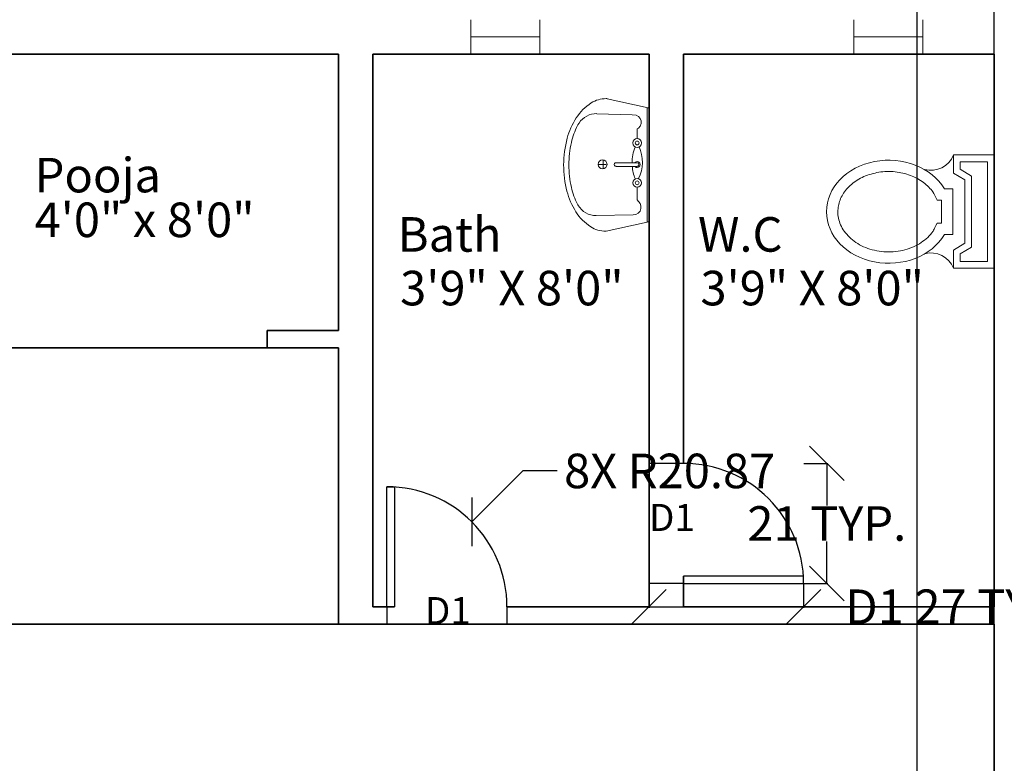
# Model space of a CAD drawing. Units: inches. Extents: x -1198 to -69, y -512 to 437.
# Tile 24 of 50: x -867 to -696, y 134 to 263. Entities that reach past the tile are written whole.
import ezdxf

# ---------------------------------------------------------------- set-up
doc = ezdxf.new("R2010")
doc.units = ezdxf.units.IN
doc.header["$MEASUREMENT"] = 0
for name, color, linetype, lineweight in [('A-ANNO-DIMS', 2, 'Continuous', 18), ('A-ANNO-SYMB', 7, 'Continuous', 18), ('A-AREA-IDEN', 7, 'Continuous', 18), ('A-FLOR-FIXT', 60, 'Continuous', 18), ('A-WALL', 7, 'Continuous', 35), ('Doors', 140, 'Continuous', 25), ('windows', 160, 'Continuous', 18)]:
    doc.layers.add(name, color=color, linetype=linetype, lineweight=lineweight)
doc.styles.get("Standard").update_dxf_attribs({"font": 'arial.ttf'})
doc.dimstyles.get("Standard").update_dxf_attribs({"dimtxt": 6, "dimasz": 6, "dimexe": 0.18, "dimexo": 0.0625, "dimgap": 0.09, "dimtad": 0, "dimtih": 1, "dimtoh": 1, "dimdec": 0, "dimzin": 0, "dimdsep": 46, "dimlunit": 4, "dimtxsty": 'Standard', "dimblk": 'OBLIQUE', "dimcen": 0.09, "dimadec": 0, "dimazin": 0, "dimtfac": 1, "dimtdec": 0, "dimtofl": 0, "dimtmove": 0, "dimatfit": 3, "dimfxl": 1, "dimtolj": 1, "dimtzin": 0, "dimarcsym": 0})

# ---------------------------------------------------------------- blocks, each defined once
blk = doc.blocks.new('A$C7C8779AE')
for p, q in [((0, 0.7405), (0, 0.5605)), ((0.5, 0.7405), (0, 0.7405)), ((0.5, 0.5605), (0.5, 0.7405)), ((0.47, 0.7105), (0.03, 0.7105)), ((0.03, 0.7105), (0.03, 0.5905)), ((0.47, 0.5905), (0.47, 0.7105)), ((0.093, 0.6405), (0.063, 0.5905)), ((0.11, 0.6105), (0.08, 0.5605)), ((0.093, 0.6405), (0.407, 0.6405)), ((0.11, 0.6105), (0.39, 0.6105)), ((0.42, 0.5605), (0.39, 0.6105)), ((0.437, 0.5905), (0.407, 0.6405)), ((0.03, 0.5905), (0.063, 0.5905)), ((0.437, 0.5905), (0.47, 0.5905)), ((0, 0.5605), (0.08, 0.5605)), ((0.1497, 0.557), (0.1497, 0.5203)), ((0.1497, 0.557), (0.3514, 0.557)), ((0.3514, 0.557), (0.3514, 0.5203)), ((0.42, 0.5605), (0.5, 0.5605)), ((0.1997, 0.507), (0.1997, 0.4879)), ((0.1997, 0.507), (0.3014, 0.507)), ((0.3014, 0.507), (0.3014, 0.4879))]:
    blk.add_line(p, q)
for centre, start, end in [((-0.0386, 0.4613), 344.642, 68.7339), ((0.5386, 0.4613), 111.2661, 195.358)]:
    blk.add_arc(centre, 0.1064, start, end)
blk.add_ellipse((0.2506, 0.2744), major_axis=(0, 0.2744), ratio=0.828948, start_param=0.459479, end_param=5.823706)
blk.add_open_spline([(0.1997, 0.4879), (0.1697, 0.474), (0.1642, 0.4702), (0.1512, 0.4602), (0.1438, 0.4535), (0.1298, 0.4388), (0.1233, 0.4306), (0.1111, 0.4131), (0.1055, 0.4037), (0.0956, 0.3838), (0.0912, 0.3733), (0.0838, 0.3516), (0.0808, 0.3403), (0.0762, 0.3172), (0.0746, 0.3055), (0.073, 0.2817), (0.0729, 0.2698), (0.0743, 0.246), (0.0758, 0.2342), (0.0801, 0.2111), (0.0831, 0.1998), (0.0903, 0.1779), (0.0945, 0.1673), (0.1043, 0.1473), (0.1098, 0.1378), (0.1218, 0.12), (0.1283, 0.1118), (0.1421, 0.0968), (0.1494, 0.09), (0.1646, 0.078), (0.1725, 0.0728), (0.1887, 0.064), (0.1969, 0.0603), (0.2137, 0.0547), (0.2222, 0.0527), (0.2392, 0.0502), (0.2478, 0.0498), (0.2664, 0.0505), (0.2764, 0.052), (0.2963, 0.0573), (0.3061, 0.061), (0.3253, 0.0707), (0.3346, 0.0766), (0.3525, 0.0906), (0.3611, 0.0987), (0.3771, 0.1169), (0.3845, 0.127), (0.3978, 0.1488), (0.4037, 0.1605), (0.4137, 0.1853), (0.4178, 0.1983), (0.424, 0.2251), (0.4261, 0.2389), (0.4282, 0.2668), (0.4283, 0.2809), (0.4262, 0.3088), (0.4241, 0.3226), (0.418, 0.3495), (0.414, 0.3625), (0.404, 0.3873), (0.3982, 0.3991), (0.385, 0.421), (0.3776, 0.4311), (0.3617, 0.4494), (0.3531, 0.4575), (0.3382, 0.4693), (0.3321, 0.4736), (0.3014, 0.4879)], degree=3, knots=[0.459479, 0.459479, 0.459479, 0.459479, 0.567422, 0.567422, 0.720865, 0.720865, 0.874307, 0.874307, 1.02775, 1.02775, 1.181192, 1.181192, 1.334635, 1.334635, 1.488077, 1.488077, 1.64152, 1.64152, 1.794963, 1.794963, 1.948405, 1.948405, 2.101848, 2.101848, 2.25529, 2.25529, 2.408733, 2.408733, 2.562175, 2.562175, 2.715618, 2.715618, 2.86906, 2.86906, 3.022503, 3.022503, 3.175946, 3.175946, 3.356457, 3.356457, 3.536968, 3.536968, 3.717479, 3.717479, 3.89799, 3.89799, 4.078501, 4.078501, 4.259012, 4.259012, 4.439523, 4.439523, 4.620035, 4.620035, 4.800546, 4.800546, 4.981057, 4.981057, 5.161568, 5.161568, 5.342079, 5.342079, 5.52259, 5.52259, 5.703101, 5.703101, 5.823706, 5.823706, 5.823706, 5.823706])
blk = doc.blocks.new('A')
at = {"xscale": 1000, "yscale": 1000, "zscale": 1000}
blk.add_blockref('A$C7C8779AE', (-250.6, 0), dxfattribs=at)
blk = doc.blocks.new('A$C6AA41FE3')
at = {"linetype": 'ByBlock'}
for p, q in [((0.1919, 0.5849), (0.3733, 0.5439)), ((0.3687, 0.04), (0.3687, 0.5439)), ((0.3687, 0.5439), (0.3772, 0.5439)), ((0.3772, 0.0411), (0.3772, 0.5439)), ((0.3026, 0.514), (0.1469, 0.5187)), ((0.32, 0.5127), (0.3026, 0.514)), ((0.3305, 0.5069), (0.32, 0.5127)), ((0.3383, 0.4979), (0.3305, 0.5069)), ((0.3425, 0.4869), (0.3383, 0.4979)), ((0.3425, 0.4752), (0.3425, 0.4869)), ((0.3251, 0.409), (0.3253, 0.4524)), ((0.3253, 0.4524), (0.3305, 0.4553)), ((0.3305, 0.4553), (0.3383, 0.4642)), ((0.3383, 0.4642), (0.3425, 0.4752)), ((0.1747, 0.3146), (0.1747, 0.2774)), ((0.1525, 0.2951), (0.1884, 0.2951)), ((0.2326, 0.3025), (0.3243, 0.3025)), ((0.2326, 0.3021), (0.2326, 0.3025)), ((0.2326, 0.2863), (0.2326, 0.2867)), ((0.3243, 0.2863), (0.2326, 0.2863)), ((0.3243, 0.3025), (0.3243, 0.3024)), ((0.3243, 0.2864), (0.3243, 0.2863)), ((0.3243, 0.1379), (0.3245, 0.1941)), ((0.3374, 0.1229), (0.3243, 0.1379)), ((0.3296, 0.0802), (0.3374, 0.0892)), ((0.3415, 0.1119), (0.3374, 0.1229)), ((0.3374, 0.0892), (0.3415, 0.1002)), ((0.3415, 0.1002), (0.3415, 0.1119)), ((0.144, 0.0693), (0.3071, 0.0724)), ((0.3071, 0.0724), (0.3191, 0.0744)), ((0.3191, 0.0744), (0.3296, 0.0802)), ((0.188, 0), (0.3687, 0.04)), ((0.3772, 0.0411), (0.3687, 0.0411))]:
    blk.add_line(p, q, dxfattribs=at)
for centre, radius in [((0.3245, 0.3895), 0.0195), ((0.3245, 0.3895), 0.00849), ((0.172, 0.2951), 0.0195), ((0.3245, 0.2136), 0.0195), ((0.3245, 0.2136), 0.00849)]:
    blk.add_circle(centre, radius, dxfattribs=at)
for centre, radius, start, end in [((0.241, 0.3799), 0.2208, 122.6461, 147.0936), ((0.1864, 0.4671), 0.118, 89.1785, 123.1413), ((0.1877, 0.4667), 0.1183, 87.9266, 89.8113), ((0.3304, 0.324), 0.3262, 147.383, 164.6821), ((0.1441, 0.4288), 0.09, 88.2595, 147.7588), ((0.3272, 0.3256), 0.3003, 152.1306, 167.3001), ((0.2193, 0.3814), 0.1789, 147.7588, 151.7723), ((0.4743, 0.289), 0.4743, 165.1956, 179.4863), ((0.5, 0.2906), 0.4766, 167.7656, 179.7702), ((0.4839, 0.3016), 0.1818, 157.4645, 179.7061), ((0.1798, 0.3042), 0.1678, 334.4875, 24.1794), ((0.3243, 0.2944), 0.013, 218.4979, 141.5021), ((0.3243, 0.2944), 0.0134, 270, 90), ((0.4743, 0.2935), 0.4743, 180.0316, 194.3223), ((0.5, 0.2944), 0.4766, 180.2298, 192.2344), ((0.2312, 0.2944), 0.0078, 80.1551, 279.8449), ((0.4839, 0.3016), 0.1818, 184.8087, 202.5355), ((0.3243, 0.2944), 0.00798, 270, 90), ((0.33, 0.2597), 0.3262, 194.841, 212.14), ((0.3272, 0.2594), 0.3003, 192.6999, 207.8694), ((0.2193, 0.2037), 0.1789, 208.2281, 209.9799), ((0.1423, 0.1592), 0.09, 209.9799, 271.0537), ((0.2402, 0.2046), 0.2208, 212.4413, 236.8887), ((0.1848, 0.1179), 0.1179, 236.4084, 270.3713), ((0.1861, 0.1183), 0.1183, 269.7541, 270.9471)]:
    blk.add_arc(centre, radius, start, end, dxfattribs=at)
blk = doc.blocks.new('A1')
at = {"xscale": 1000, "yscale": 1000, "zscale": 1000, "rotation": 90}
blk.add_blockref('A$C6AA41FE3', (292.5, -377.2), dxfattribs=at)
blk = doc.blocks.new('VENT-12')
at = {"ltscale": 10}
for p, q in [((0, 6), (0, 0)), ((12, 6), (12, 0)), ((0, 3), (12, 3))]:
    blk.add_line(p, q, dxfattribs=at)
blk = doc.blocks.new('DOOR-D1-JAMB3')
for p, q in [((0, 0), (0, -3)), ((20.87, 0), (20.87, -3))]:
    blk.add_line(p, q)
blk.add_lwpolyline([(0, 0), (0, 20.87), (1.3, 20.87), (1.3, 0)], close=True)
blk.add_arc((0, 0), 20.87, 0, 90)
blk = doc.blocks.new('DOOR-D1-JAMB6')
for p, q in [((0, 20.87), (-6, 20.87)), ((0, 0), (-6, 0))]:
    blk.add_line(p, q)
blk.add_lwpolyline([(0, 0), (20.87, 0), (20.87, 1.3), (0, 1.3)], close=True)
blk.add_arc((0, 0), 20.87, 0, 90)
blk = doc.blocks.new('_Oblique')
at = {"color": 0, "linetype": 'ByBlock', "lineweight": -2}
blk.add_line((-0.5, -0.5), (0.5, 0.5), dxfattribs=at)
blk = doc.blocks.new('*D34')
at = {"layer": 'A-ANNO-DIMS', "color": 0, "lineweight": -2, "ltscale": 10, "transparency": 16777216}
for p, q in [((-757.75, 165.22), (-757.75, 161.07)), ((-730.88, 165.22), (-730.88, 161.07)), ((-757.75, 161.25), (-730.88, 161.25)), ((-730.88, 161.25), (-724.88, 161.25))]:
    blk.add_line(p, q, dxfattribs=at)
at = {"layer": 'DEFPOINTS', "color": 0, "ltscale": 10, "transparency": 16777216}
for p in [(-757.75, 165.28), (-730.88, 165.28), (-730.88, 161.25)]:
    blk.add_point(p, dxfattribs=at)
at = {"layer": 'A-ANNO-DIMS', "color": 0, "lineweight": -2, "ltscale": 10, "transparency": 16777216, "xscale": 6, "yscale": 6, "zscale": 6, "rotation": 180}
blk.add_blockref('_Oblique', (-757.75, 161.25), dxfattribs=at)
at = {"layer": 'A-ANNO-DIMS', "color": 0, "lineweight": -2, "ltscale": 10, "transparency": 16777216, "xscale": 6, "yscale": 6, "zscale": 6}
blk.add_blockref('_Oblique', (-730.88, 161.25), dxfattribs=at)
at = {"layer": 'A-ANNO-DIMS', "color": 0, "ltscale": 10, "transparency": 16777216, "insert": (-703.82, 161.25), "char_height": 6, "attachment_point": 5}
blk.add_mtext('\\A1;D1 27 TYP.', dxfattribs=at)
blk = doc.blocks.new('*D35')
at = {"layer": 'A-ANNO-DIMS', "color": 0, "lineweight": -2, "ltscale": 10, "transparency": 16777216}
for p, q in [((-730.82, 186.15), (-726.67, 186.15)), ((-726.85, 186.15), (-726.85, 178.82)), ((-726.85, 165.28), (-726.85, 172.61)), ((-730.82, 165.28), (-726.67, 165.28))]:
    blk.add_line(p, q, dxfattribs=at)
at = {"layer": 'DEFPOINTS', "color": 0, "ltscale": 10, "transparency": 16777216}
for p in [(-730.88, 186.15), (-726.85, 186.15), (-730.88, 165.28)]:
    blk.add_point(p, dxfattribs=at)
at = {"layer": 'A-ANNO-DIMS', "color": 0, "lineweight": -2, "ltscale": 10, "transparency": 16777216, "xscale": 6, "yscale": 6, "zscale": 6}
for p, rotation in [((-726.85, 186.15), 90), ((-726.85, 165.28), 270)]:
    blk.add_blockref('_Oblique', p, dxfattribs=dict(at, rotation=rotation))
at = {"layer": 'A-ANNO-DIMS', "color": 0, "ltscale": 10, "transparency": 16777216, "insert": (-726.85, 175.71), "char_height": 6, "attachment_point": 5}
blk.add_mtext('\\A1;21 TYP.', dxfattribs=at)
blk = doc.blocks.new('*D76')
at = {"layer": 'A-ANNO-DIMS', "color": 0, "lineweight": -2, "ltscale": 10, "transparency": 16777216}
for p, q in [((-711.13, -38.21), (-711.13, 433.18)), ((-697.75, -38.21), (-697.75, 433.18)), ((-711.13, 433), (-697.75, 433)), ((-697.75, 433), (-691.75, 433))]:
    blk.add_line(p, q, dxfattribs=at)
at = {"layer": 'DEFPOINTS', "color": 0, "ltscale": 10, "transparency": 16777216}
for p in [(-697.75, 433), (-711.13, -38.27), (-697.75, -38.27)]:
    blk.add_point(p, dxfattribs=at)
at = {"layer": 'A-ANNO-DIMS', "color": 0, "lineweight": -2, "ltscale": 10, "transparency": 16777216, "xscale": 6, "yscale": 6, "zscale": 6, "rotation": 180}
blk.add_blockref('_Oblique', (-711.13, 433), dxfattribs=at)
at = {"layer": 'A-ANNO-DIMS', "color": 0, "lineweight": -2, "ltscale": 10, "transparency": 16777216, "xscale": 6, "yscale": 6, "zscale": 6}
blk.add_blockref('_Oblique', (-697.75, 433), dxfattribs=at)
at = {"layer": 'A-ANNO-DIMS', "color": 0, "ltscale": 10, "transparency": 16777216, "insert": (-681.81, 433), "char_height": 6, "attachment_point": 5}
blk.add_mtext('\\A1;13.38', dxfattribs=at)
blk = doc.blocks.new('*D83')
at = {"layer": 'A-ANNO-DIMS', "color": 0, "lineweight": -2, "ltscale": 10, "transparency": 16777216}
for p, q in [((-779.71, 184.84), (-788.56, 175.99)), ((-773.71, 184.84), (-779.71, 184.84)), ((-803.41, 161.23), (-803.23, 161.23)), ((-803.32, 161.14), (-803.32, 161.32))]:
    blk.add_line(p, q, dxfattribs=at)
at = {"layer": 'DEFPOINTS', "color": 0, "ltscale": 10, "transparency": 16777216}
for p in [(-788.56, 175.99), (-803.32, 161.23)]:
    blk.add_point(p, dxfattribs=at)
at = {"layer": 'A-ANNO-DIMS', "color": 0, "lineweight": -2, "ltscale": 10, "transparency": 16777216, "xscale": 6, "yscale": 6, "zscale": 6, "rotation": 225.0010987737688}
blk.add_blockref('_Oblique', (-788.56, 175.99), dxfattribs=at)
at = {"layer": 'A-ANNO-DIMS', "color": 0, "ltscale": 10, "transparency": 16777216, "insert": (-754.17, 184.84), "char_height": 6, "attachment_point": 5}
blk.add_mtext('\\A1;8X R20.87', dxfattribs=at)

msp = doc.modelspace()

# ---------------------------------------------------------------- linework, layer by layer
at = {"layer": 'A-WALL', "ltscale": 10}
for p, q in [((-811.7509, 257.2277), (-886.7509, 257.2277)), ((-811.7509, 257.2277), (-811.7509, 209.2277)), ((-805.7509, 257.2277), (-805.7509, 161.2277)), ((-757.7509, 257.2277), (-805.7509, 257.2277)), ((-757.7509, 257.2277), (-757.7509, 161.2277)), ((-697.7509, 257.2277), (-751.7509, 257.2277)), ((-751.7509, 257.2277), (-751.7509, 186.149)), ((-697.7509, 257.2277), (-697.7509, 161.2277)), ((-811.7509, 209.2277), (-824.1219, 209.2277)), ((-824.1219, 209.2277), (-824.1219, 206.2277)), ((-811.7509, 206.2277), (-892.7509, 206.2277)), ((-811.7509, 206.2277), (-811.7509, 161.2277)), ((-751.7509, 166.5837), (-751.7509, 161.2277)), ((-811.7509, 161.2277), (-811.7509, 158.2277)), ((-802.0154, 161.2277), (-805.7509, 161.2277)), ((-757.7509, 161.2277), (-782.4501, 161.2277)), ((-697.7509, 161.2277), (-751.7509, 161.2277)), ((-697.7509, 158.2277), (-886.7509, 158.2277)), ((-697.7509, 158.2277), (-697.7509, 35.2277))]:
    msp.add_line(p, q, dxfattribs=at)

# ---------------------------------------------------------------- block references
at = {"layer": 'A-FLOR-FIXT', "ltscale": 10, "xscale": 0.0393700787401575, "yscale": 0.0393700787401575, "zscale": 0.0393700787401575, "rotation": 270}
for name, p in [('A1', (-757.7509, 237.9979)), ('A', (-726.9029, 229.8684))]:
    msp.add_blockref(name, p, dxfattribs=at)
at = {"layer": 'Doors'}
for name, p in [('DOOR-D1-JAMB6', (-751.7509, 165.2794)), ('DOOR-D1-JAMB3', (-803.3198, 161.2277)), ('DOOR-D1-JAMB3', (-803.3198, 161.2277))]:
    msp.add_blockref(name, p, dxfattribs=at)
at = {"layer": 'windows', "rotation": 180}
msp.add_blockref('VENT-12', (-776.7361, 263.2273), dxfattribs=at)
at = {"layer": 'windows'}
msp.add_blockref('VENT-12', (-722.179, 257.228), dxfattribs=at)

# ---------------------------------------------------------------- texts
at = {"layer": 'A-ANNO-SYMB', "ltscale": 10}
for p in [(-757.7509, 174.4049), (-796.7071, 158.2277)]:
    msp.add_text('D1', height=4.69957, dxfattribs=at).set_placement(p)
at = {"layer": 'A-AREA-IDEN', "ltscale": 10, "char_height": 6, "attachment_point": 1}
for s, insert in [('Pooja', (-864.5573, 239.2277)), ('4\'0" x 8\'0"', (-864.5573, 231.4637)), ('Bath', (-801.4421, 228.9301)), ('W.C', (-749.2349, 228.9301)), ('3\'9" X 8\'0"', (-801.0227, 219.603)), ('3\'9" X 8\'0"', (-748.8154, 219.603))]:
    msp.add_mtext_dynamic_manual_height_columns(s, width=57.976527, gutter_width=30, heights=[0], dxfattribs=dict(at, insert=insert))

# ---------------------------------------------------------------- dimensions: what is measured, and where the dimension line sits
at = {"layer": 'A-ANNO-DIMS', "ltscale": 10}
dim = msp.add_linear_dim(base=(-697.7509, 433.0036), p1=(-711.1319, -38.2723), p2=(-697.7509, -38.2723), dimstyle='Standard', override={"dimdec": 2, "dimlfac": 1, "dimrnd": 0, "dimzin": 0, "dimdsep": 46, "dimlunit": 2}, dxfattribs=at)
dim.commit()
dim.dimension.update_dxf_attribs({"geometry": '*D76', "text_midpoint": (-681.8137, 433.0036)})
dim = msp.add_radius_dim(center=(-803.3198, 161.2277), mpoint=(-788.563, 175.985), text='8X <>', dimstyle='Standard', override={"dimdec": 2, "dimlfac": 1, "dimrnd": 0, "dimzin": 0, "dimdsep": 46, "dimlunit": 2}, dxfattribs=at)
dim.commit()
dim.dimension.update_dxf_attribs({"geometry": '*D83', "text_midpoint": (-754.1741, 184.8395), "dimtype": 164})
dim = msp.add_linear_dim(base=(-726.8507, 186.149), p1=(-730.8812, 165.2794), p2=(-730.8812, 186.149), angle=90, text='<> TYP.', dimstyle='Standard', override={"dimdec": 0, "dimlfac": 1, "dimrnd": 0, "dimzin": 0, "dimdsep": 46, "dimlunit": 2}, dxfattribs=at)
dim.commit()
dim.dimension.update_dxf_attribs({"geometry": '*D35', "text_midpoint": (-726.8507, 175.7142)})
dim = msp.add_linear_dim(base=(-730.8812, 161.2489), p1=(-757.7509, 165.2794), p2=(-730.8812, 165.2794), text='D1 <> TYP.', dimstyle='Standard', override={"dimdec": 0, "dimlfac": 1, "dimrnd": 0, "dimzin": 0, "dimdsep": 46, "dimlunit": 2}, dxfattribs=at)
dim.commit()
dim.dimension.update_dxf_attribs({"geometry": '*D34', "text_midpoint": (-703.8157, 161.2489)})

doc.saveas('drawing.dxf')
